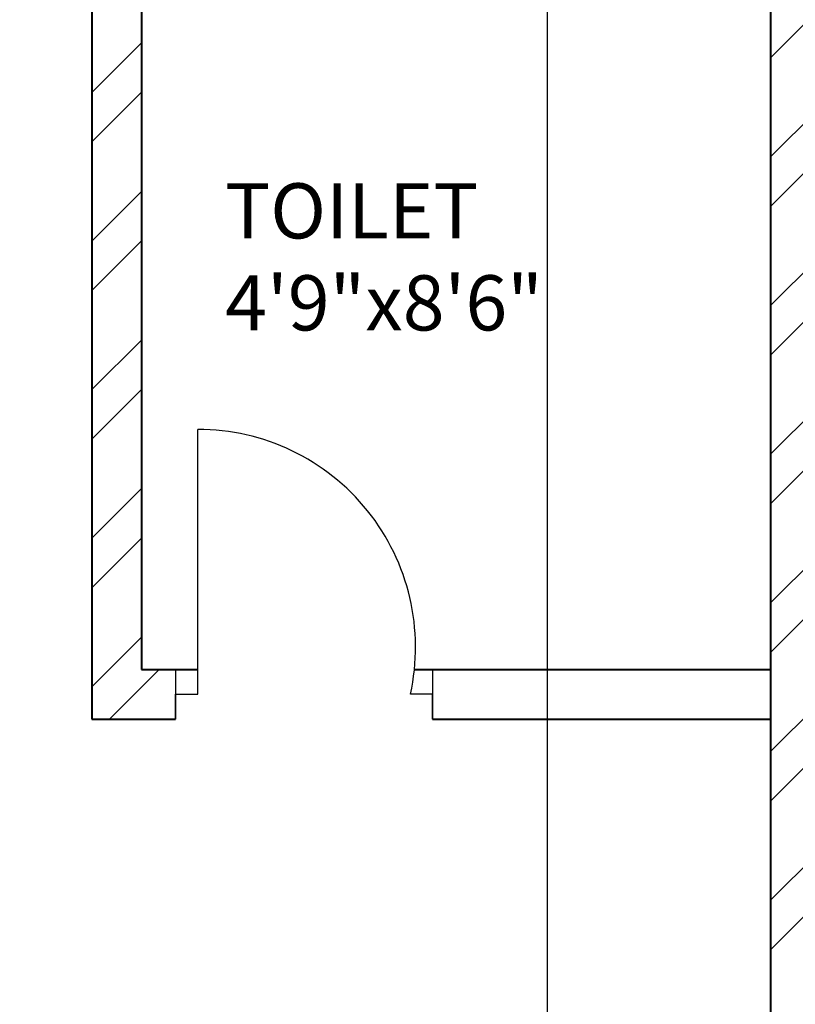
# Model space of a CAD drawing. Units: inches. Extents: x 1601 to 2297, y 1496 to 2631.
# Tile 43 of 57: x 1820 to 1891, y 2391 to 2480. Entities that reach past the tile are written whole.
import ezdxf

# ---------------------------------------------------------------- set-up
doc = ezdxf.new("R2010")
doc.units = ezdxf.units.IN
for name, color, linetype, lineweight in [('A-ANNO-DIMS', 2, 'Continuous', 18), ('A-AREA-IDEN', 7, 'Continuous', 18), ('A-DOOR', 21, 'Continuous', 25), ('A-WALL', 7, 'Continuous', 40), ('A-WALL-PATT', 215, 'Continuous', 13)]:
    doc.layers.add(name, color=color, linetype=linetype, lineweight=lineweight)
doc.styles.get("Standard").update_dxf_attribs({"font": 'arial.ttf'})
doc.dimstyles.get("Standard").update_dxf_attribs({"dimtxt": 0.18, "dimasz": 0.18, "dimexe": 0.18, "dimexo": 0.0625, "dimgap": 0.09, "dimtad": 0, "dimtih": 1, "dimtoh": 1, "dimdec": 4, "dimzin": 0, "dimdsep": 46, "dimtxsty": 'Standard', "dimcen": 0.09, "dimadec": 0, "dimazin": 0, "dimtfac": 1, "dimtdec": 4, "dimtofl": 0, "dimtmove": 0, "dimatfit": 3, "dimfxl": 1, "dimtolj": 1, "dimtzin": 0, "dimarcsym": 0})

# ---------------------------------------------------------------- blocks, each defined once
blk = doc.blocks.new('*D33')
at = {"layer": 'A-ANNO-DIMS', "color": 0, "lineweight": -2, "transparency": 16777216}
for p, q in [((1764.337, 2136.388), (1764.337, 2581.055)), ((1764.517, 2580.875), (1816.057, 2580.875)), ((1868.157, 2580.875), (1816.617, 2580.875)), ((1868.337, 2136.388), (1868.337, 2581.055))]:
    blk.add_line(p, q, dxfattribs=at)
at = {"layer": 'A-ANNO-DIMS', "color": 0, "transparency": 16777216}
for points in [[(1764.517, 2580.905), (1764.517, 2580.845), (1764.337, 2580.875)], [(1868.157, 2580.905), (1868.157, 2580.845), (1868.337, 2580.875)]]:
    blk.add_solid(points, dxfattribs=at)
at = {"layer": 'Defpoints', "color": 0, "transparency": 16777216}
for p in [(1868.337, 2580.875), (1764.337, 2136.325), (1868.337, 2136.325)]:
    blk.add_point(p, dxfattribs=at)
at = {"layer": 'A-ANNO-DIMS', "color": 0, "transparency": 16777216, "insert": (1816.337, 2580.875), "char_height": 0.18, "attachment_point": 5}
blk.add_mtext('\\A1;104', dxfattribs=at)

msp = doc.modelspace()

# ---------------------------------------------------------------- hatches: boundary and pattern name
at = {"layer": 'A-WALL-PATT'}
h = msp.add_hatch(dxfattribs=at)
h.set_pattern_fill('ANSI32', color=256)
h.paths.add_polyline_path([(1842.0336, 2528.0767), (1842.0336, 2532.3254), (1686.0373, 2532.3254), (1686.0373, 2492.9493), (1695.0373, 2492.9493), (1695.0373, 2523.3254), (1827.0373, 2523.3254), (1827.0373, 2416.8254), (1834.6225, 2416.8254), (1834.6225, 2419.0754), (1834.6225, 2421.3254), (1831.5373, 2421.3254), (1831.5373, 2523.3254), (1842.0336, 2523.3254)])
h.paths.add_polyline_path([(1695.0373, 2432.9493), (1686.0373, 2432.9493), (1686.0373, 2325.989), (1695.0373, 2325.989), (1695.0373, 2347.8254), (1827.0373, 2347.8254), (1827.0373, 2287.8254), (1823.2991, 2287.8254), (1823.2991, 2283.3254), (1847.9422, 2283.3254), (1847.9422, 2285.5754), (1847.9422, 2287.8254), (1831.5373, 2287.8254), (1831.5373, 2347.8254), (1846.9946, 2347.8254), (1846.9946, 2350.0754), (1846.9946, 2352.3254), (1695.0373, 2352.3254)])
h.paths.add_polyline_path([(1807.1169, 1573.5395), (2055.0405, 1573.5395), (2055.0405, 1610.6322), (1807.1169, 1610.6322)], flags=9)
h.paths.add_polyline_path([(1841.1631, 1712.7967), (1870.3957, 1712.7967), (1870.3957, 1731.454), (1841.1631, 1731.454)], flags=9)
h.paths.add_polyline_path([(2144.3862, 1772.185), (2191.0233, 1772.185), (2191.0233, 1790.8423), (2144.3862, 1790.8423)], flags=9)
h.paths.add_polyline_path([(2143.0128, 1827.3312), (2177.9958, 1827.3312), (2177.9958, 1845.9886), (2143.0128, 1845.9886)], flags=9)
h.paths.add_polyline_path([(2041.2439, 1833.5691), (2070.8516, 1833.5691), (2070.8516, 1852.2264), (2041.2439, 1852.2264)], flags=9)
h.paths.add_polyline_path([(2097.2791, 1947.0598), (2134.2061, 1947.0598), (2134.2061, 1965.7171), (2097.2791, 1965.7171)], flags=9)
h.paths.add_polyline_path([(2214.995, 1904.3124), (2214.995, 1942.2899), (2196.3376, 1942.2899), (2196.3376, 1904.3124)], flags=9)
h.paths.add_polyline_path([(2186.6284, 2043.8031), (2219.7935, 2043.8031), (2219.7935, 2062.4605), (2186.6284, 2062.4605)], flags=9)
h.paths.add_polyline_path([(2064.0877, 2031.616), (2097.4949, 2031.616), (2097.4949, 2050.2734), (2064.0877, 2050.2734)], flags=9)
h.paths.add_polyline_path([(1973.1349, 1986.0688), (2008.4009, 1986.0688), (2008.4009, 2004.7261), (1973.1349, 2004.7261)], flags=9)
h.paths.add_polyline_path([(1976.3676, 2106.9635), (2005.7469, 2106.9635), (2005.7469, 2125.6209), (1976.3676, 2125.6209)], flags=9)
h.paths.add_polyline_path([(1991.7852, 2180.4863), (2027.0513, 2180.4863), (2027.0513, 2199.1437), (1991.7852, 2199.1437)], flags=9)
h.paths.add_polyline_path([(2106.1801, 2187.9359), (2152.2101, 2187.9359), (2152.2101, 2206.5932), (2106.1801, 2206.5932)], flags=9)
h.paths.add_polyline_path([(2148.6686, 2262.2542), (2182.318, 2262.2542), (2182.318, 2280.9115), (2148.6686, 2280.9115)], flags=9)
h.paths.add_polyline_path([(2041.6327, 2252.8147), (2071.2405, 2252.8147), (2071.2405, 2271.4721), (2041.6327, 2271.4721)], flags=9)
h.paths.add_polyline_path([(2063.9734, 2375.4265), (2100.9004, 2375.4265), (2100.9004, 2394.0839), (2063.9734, 2394.0839)], flags=9)
h.paths.add_polyline_path([(2216.4955, 2330.9748), (2216.4955, 2370.2654), (2197.8381, 2370.2654), (2197.8381, 2330.9748)], flags=9)
h.paths.add_polyline_path([(2179.1416, 2485.8687), (2212.3067, 2485.8687), (2212.3067, 2504.5261), (2179.1416, 2504.5261)], flags=9)
h.paths.add_polyline_path([(2078.7442, 2471.1516), (2112.1514, 2471.1516), (2112.1514, 2489.809), (2078.7442, 2489.809)], flags=9)
h.paths.add_polyline_path([(1915.9631, 2329.4668), (1952.8902, 2329.4668), (1952.8902, 2348.1241), (1915.9631, 2348.1241)], flags=9)
h.paths.add_polyline_path([(1904.3189, 2499.6709), (1940.4512, 2499.6709), (1940.4512, 2518.3282), (1904.3189, 2518.3282)], flags=9)
h.paths.add_polyline_path([(1892.3665, 2100.4595), (1925.6374, 2100.4595), (1925.6374, 2119.1169), (1892.3665, 2119.1169)], flags=9)
h.paths.add_polyline_path([(1909.2984, 1805.9631), (1946.2254, 1805.9631), (1946.2254, 1824.6205), (1909.2984, 1824.6205)], flags=9)
h.paths.add_polyline_path([(1934.6056, 1658.616), (1970.738, 1658.616), (1970.738, 1677.2733), (1934.6056, 1677.2733)], flags=9)
h.paths.add_polyline_path([(1711.2052, 1789.8902), (1750.0456, 1789.8902), (1750.0456, 1808.5476), (1711.2052, 1808.5476)], flags=9)
h.paths.add_polyline_path([(1742.7874, 1854.6743), (1771.9449, 1854.6743), (1771.9449, 1873.3317), (1742.7874, 1873.3317)], flags=9)
h.paths.add_polyline_path([(1807.3592, 1997.7912), (1850.1116, 1997.7912), (1850.1116, 2016.4486), (1807.3592, 2016.4486)], flags=9)
h.paths.add_polyline_path([(1717.4579, 2237.7844), (1760.2103, 2237.7844), (1760.2103, 2256.4417), (1717.4579, 2256.4417)], flags=9)
h.paths.add_polyline_path([(1780.9285, 2324.0623), (1810.086, 2324.0623), (1810.086, 2342.7197), (1780.9285, 2342.7197)], flags=25)
h.paths.add_polyline_path([(1837.696, 2449.2024), (1866.9286, 2449.2024), (1866.9286, 2467.8598), (1837.696, 2467.8598)], flags=9)
h.paths.add_polyline_path([(1712.7752, 2484.9404), (1751.6156, 2484.9404), (1751.6156, 2503.5977), (1712.7752, 2503.5977)], flags=25)
h = msp.add_hatch(dxfattribs=at)
h.set_pattern_fill('ANSI32', color=256)
h.paths.add_polyline_path([(2230.5373, 2532.3254), (2106.0595, 2532.3254), (2106.0595, 2523.3254), (2169.0373, 2523.3254), (2169.0373, 2424.3254), (2091.3989, 2424.3254), (2091.3989, 2419.8254), (2169.0373, 2419.8254), (2169.0373, 2408.1385), (2178.0373, 2408.1385), (2178.0373, 2419.8254), (2181.0581, 2419.8254), (2181.0581, 2422.0754), (2181.0581, 2424.3254), (2178.0373, 2424.3254), (2178.0373, 2523.3254), (2226.0373, 2523.3254), (2226.0373, 2424.3254), (2206.6251, 2424.3254), (2206.6251, 2419.8254), (2226.0373, 2419.8254), (2226.0373, 2299.8254), (2226.0373, 2295.3254), (2178.0373, 2295.3254), (2178.0373, 2312.1385), (2169.0373, 2312.1385), (2169.0373, 2295.3254), (2130.0373, 2295.3254), (2130.0373, 2279.1364), (2128.0593, 2279.1364), (2128.0593, 2274.6364), (2130.0373, 2274.6364), (2130.0373, 2260.7505), (2134.5373, 2260.7505), (2134.5373, 2290.8254), (2226.0373, 2290.8254), (2226.0373, 2279.2475), (2230.5373, 2279.2475), (2230.5373, 2347.8254)])
h.paths.add_polyline_path([(2070.0595, 2532.3254), (2031.0373, 2532.3254), (2031.0373, 2466.3254), (2003.9878, 2466.3254), (2003.9878, 2457.3254), (2031.0373, 2457.3254), (2031.0373, 2419.8254), (2031.0373, 2373.1914), (2035.5373, 2373.1914), (2035.5373, 2419.8254), (2047.3393, 2419.8254), (2047.3393, 2424.3254), (2035.5373, 2424.3254), (2035.5373, 2523.3254), (2070.0595, 2523.3254), (2070.0595, 2527.8254)])
h.paths.add_polyline_path([(1893.0373, 2532.3254), (1866.0336, 2532.3254), (1866.0336, 2523.3254), (1888.5373, 2523.3254), (1888.5373, 2347.8254), (1893.0373, 2347.8254), (1893.0373, 2457.3254), (1907.9878, 2457.3254), (1907.9878, 2466.3254), (1893.0373, 2466.3254)])
h = msp.add_hatch(dxfattribs=at)
h.set_pattern_fill('ANSI32', color=256)
h.paths.add_polyline_path([(1973.9371, 2211.3254), (1893.0373, 2211.3254), (1893.0373, 2287.8254), (1884.6167, 2287.8254), (1884.6167, 2285.5754), (1884.6167, 2283.3254), (1888.5373, 2283.3254), (1888.5373, 2145.3254), (1695.0373, 2145.3254), (1695.0373, 2173.8724), (1690.5373, 2173.8724), (1686.0373, 2173.8724), (1686.0373, 2136.3254), (1722.5687, 2136.3254), (1722.5687, 2117.4352), (1731.5687, 2117.4352), (1731.5687, 2136.3254), (1893.0373, 2136.3254), (1893.0373, 2202.3254), (1959.0373, 2202.3254), (1959.0373, 2182.1303), (1968.0373, 2182.1303), (1968.0373, 2202.3254), (1973.9371, 2202.3254)])
h.paths.add_polyline_path([(2094.0373, 2274.6364), (2096.4294, 2274.6364), (2096.4294, 2276.8864), (2096.4294, 2279.1364), (2094.0373, 2279.1364), (2094.0373, 2290.8254), (2094.0373, 2295.3254), (2089.5373, 2295.3254), (2089.5373, 2230.8254), (2035.5373, 2230.8254), (2035.5373, 2299.8254), (2031.0373, 2299.8254), (2031.0373, 2211.3254), (2023.0065, 2211.3254), (2023.0065, 2202.3254), (2031.0373, 2202.3254), (2031.0373, 2140.8254), (1968.0373, 2140.8254), (1968.0373, 2145.9106), (1963.5373, 2145.9106), (1959.0373, 2145.9106), (1959.0373, 2116.839), (1963.5373, 2116.839), (1968.0373, 2116.839), (1968.0373, 2131.8254), (2031.0373, 2131.8254), (2031.0373, 2094.3254), (2031.0373, 2085.3254), (2031.0373, 2056.8254), (1968.0373, 2056.8254), (1968.0373, 2070.4947), (1963.5373, 2070.4947), (1959.0373, 2070.4947), (1959.0373, 2040.3029), (1968.0373, 2040.3029), (1968.0373, 2047.8254), (2031.0373, 2047.8254), (2031.0373, 1983.3254), (2031.0373, 1978.8254), (2021.1979, 1978.8254), (2021.1979, 1974.3254), (2031.0373, 1974.3254), (2031.0373, 1954.3528), (2035.5373, 1954.3528), (2035.5373, 1974.3254), (2035.5373, 1981.8254), (2055.5513, 1981.8254), (2055.5513, 1986.3254), (2035.5373, 1986.3254), (2035.5373, 2047.8254), (2040.0373, 2047.8254), (2040.0373, 2085.3254), (2040.0373, 2094.3254), (2040.0373, 2140.8254), (2035.5373, 2140.8254), (2035.5373, 2226.3254), (2089.5373, 2226.3254), (2094.0373, 2226.3254)])
h.paths.add_polyline_path([(2226.0373, 2230.8254), (2134.5373, 2230.8254), (2134.5373, 2233.5437), (2130.0373, 2233.5437), (2130.0373, 2226.3254), (2134.5373, 2226.3254), (2226.0373, 2226.3254)])
h.paths.add_polyline_path([(1807.1169, 1573.5395), (2055.0405, 1573.5395), (2055.0405, 1610.6322), (1807.1169, 1610.6322)], flags=9)
h.paths.add_polyline_path([(1841.1631, 1712.7967), (1870.3957, 1712.7967), (1870.3957, 1731.454), (1841.1631, 1731.454)], flags=9)
h.paths.add_polyline_path([(2144.3862, 1772.185), (2191.0233, 1772.185), (2191.0233, 1790.8423), (2144.3862, 1790.8423)], flags=9)
h.paths.add_polyline_path([(2143.0128, 1827.3312), (2177.9958, 1827.3312), (2177.9958, 1845.9886), (2143.0128, 1845.9886)], flags=9)
h.paths.add_polyline_path([(2041.2439, 1833.5691), (2070.8516, 1833.5691), (2070.8516, 1852.2264), (2041.2439, 1852.2264)], flags=9)
h.paths.add_polyline_path([(2097.2791, 1947.0598), (2134.2061, 1947.0598), (2134.2061, 1965.7171), (2097.2791, 1965.7171)], flags=9)
h.paths.add_polyline_path([(2214.995, 1904.3124), (2214.995, 1942.2899), (2196.3376, 1942.2899), (2196.3376, 1904.3124)], flags=9)
h.paths.add_polyline_path([(2186.6284, 2043.8031), (2219.7935, 2043.8031), (2219.7935, 2062.4605), (2186.6284, 2062.4605)], flags=9)
h.paths.add_polyline_path([(2064.0877, 2031.616), (2097.4949, 2031.616), (2097.4949, 2050.2734), (2064.0877, 2050.2734)], flags=9)
h.paths.add_polyline_path([(1973.1349, 1986.0688), (2008.4009, 1986.0688), (2008.4009, 2004.7261), (1973.1349, 2004.7261)], flags=25)
h.paths.add_polyline_path([(1976.3676, 2106.9635), (2005.7469, 2106.9635), (2005.7469, 2125.6209), (1976.3676, 2125.6209)], flags=25)
h.paths.add_polyline_path([(1991.7852, 2180.4863), (2027.0513, 2180.4863), (2027.0513, 2199.1437), (1991.7852, 2199.1437)], flags=25)
h.paths.add_polyline_path([(2106.1801, 2187.9359), (2152.2101, 2187.9359), (2152.2101, 2206.5932), (2106.1801, 2206.5932)], flags=9)
h.paths.add_polyline_path([(2148.6686, 2262.2542), (2182.318, 2262.2542), (2182.318, 2280.9115), (2148.6686, 2280.9115)], flags=9)
h.paths.add_polyline_path([(2041.6327, 2252.8147), (2071.2405, 2252.8147), (2071.2405, 2271.4721), (2041.6327, 2271.4721)], flags=25)
h.paths.add_polyline_path([(2063.9734, 2375.4265), (2100.9004, 2375.4265), (2100.9004, 2394.0839), (2063.9734, 2394.0839)], flags=9)
h.paths.add_polyline_path([(2216.4955, 2330.9748), (2216.4955, 2370.2654), (2197.8381, 2370.2654), (2197.8381, 2330.9748)], flags=9)
h.paths.add_polyline_path([(2179.1416, 2485.8687), (2212.3067, 2485.8687), (2212.3067, 2504.5261), (2179.1416, 2504.5261)], flags=9)
h.paths.add_polyline_path([(2078.7442, 2471.1516), (2112.1514, 2471.1516), (2112.1514, 2489.809), (2078.7442, 2489.809)], flags=9)
h.paths.add_polyline_path([(1915.9631, 2329.4668), (1952.8902, 2329.4668), (1952.8902, 2348.1241), (1915.9631, 2348.1241)], flags=9)
h.paths.add_polyline_path([(1904.3189, 2499.6709), (1940.4512, 2499.6709), (1940.4512, 2518.3282), (1904.3189, 2518.3282)], flags=9)
h.paths.add_polyline_path([(1892.3665, 2100.4595), (1925.6374, 2100.4595), (1925.6374, 2119.1169), (1892.3665, 2119.1169)], flags=9)
h.paths.add_polyline_path([(1909.2984, 1805.9631), (1946.2254, 1805.9631), (1946.2254, 1824.6205), (1909.2984, 1824.6205)], flags=9)
h.paths.add_polyline_path([(1934.6056, 1658.616), (1970.738, 1658.616), (1970.738, 1677.2733), (1934.6056, 1677.2733)], flags=9)
h.paths.add_polyline_path([(1711.2052, 1789.8902), (1750.0456, 1789.8902), (1750.0456, 1808.5476), (1711.2052, 1808.5476)], flags=9)
h.paths.add_polyline_path([(1742.7874, 1854.6743), (1771.9449, 1854.6743), (1771.9449, 1873.3317), (1742.7874, 1873.3317)], flags=9)
h.paths.add_polyline_path([(1807.3592, 1997.7912), (1850.1116, 1997.7912), (1850.1116, 2016.4486), (1807.3592, 2016.4486)], flags=9)
h.paths.add_polyline_path([(1717.4579, 2237.7844), (1760.2103, 2237.7844), (1760.2103, 2256.4417), (1717.4579, 2256.4417)], flags=25)
h.paths.add_polyline_path([(1780.9285, 2324.0623), (1810.086, 2324.0623), (1810.086, 2342.7197), (1780.9285, 2342.7197)], flags=9)
h.paths.add_polyline_path([(1837.696, 2449.2024), (1866.9286, 2449.2024), (1866.9286, 2467.8598), (1837.696, 2467.8598)], flags=9)
h.paths.add_polyline_path([(1712.7752, 2484.9404), (1751.6156, 2484.9404), (1751.6156, 2503.5977), (1712.7752, 2503.5977)], flags=9)
h = msp.add_hatch(dxfattribs=at)
h.set_pattern_fill('ANSI32', color=256)
h.paths.add_polyline_path([(2230.5373, 1861.8254), (2182.5373, 1861.8254), (2182.5373, 1885.3637), (2178.0373, 1885.3637), (2178.0373, 1861.8254), (2166.0373, 1861.8254), (2134.5373, 1861.8254), (2130.0373, 1861.8254), (2130.0373, 1841.4682), (2126.8833, 1841.4682), (2126.8833, 1836.9682), (2130.0373, 1836.9682), (2130.0373, 1822.7302), (2134.5373, 1822.7302), (2134.5373, 1857.3254), (2166.0373, 1857.3254), (2226.0373, 1857.3254), (2226.0373, 1846.1155), (2230.5373, 1846.1155)])
h.paths.add_polyline_path([(2226.0373, 1797.3254), (2134.5373, 1797.3254), (2134.5373, 1800.6636), (2132.2873, 1800.6636), (2130.0373, 1800.6636), (2130.0373, 1797.3254), (2130.0373, 1792.8254), (2167.7264, 1792.8254), (2226.0373, 1792.8254)])
h.paths.add_polyline_path([(2230.5373, 1822.1155), (2226.0373, 1822.1155), (2226.0373, 1760.8563), (2230.5373, 1760.8563)])
h.paths.add_polyline_path([(2230.5373, 1700.8563), (2226.0373, 1700.8563), (2226.0373, 1644.3254), (2140.2517, 1644.3254), (2140.2517, 1635.3254), (2230.5373, 1635.3254)])
h.paths.add_polyline_path([(2080.2517, 1639.8254), (2080.2517, 1644.3254), (2035.5373, 1644.3254), (2035.5373, 1792.8254), (2094.0373, 1792.8254), (2094.0373, 1797.3254), (2094.0373, 1836.9682), (2097.1057, 1836.9682), (2097.1057, 1839.2182), (2097.1057, 1841.4682), (2094.0373, 1841.4682), (2094.0373, 1862.2276), (2089.5373, 1862.2276), (2089.5373, 1797.3254), (2035.5373, 1797.3254), (2035.5373, 1857.3254), (2035.5373, 1885.0916), (2031.0373, 1885.0916), (2031.0373, 1710.3254), (2012.329, 1710.3254), (2012.329, 1701.3254), (2031.0373, 1701.3254), (2031.0373, 1644.3254), (2031.0373, 1635.3254), (2080.2517, 1635.3254)])
h.paths.add_polyline_path([(1836.0373, 1653.2033), (1842.6171, 1653.2033), (1842.6171, 1657.7033), (1842.6171, 1662.2033), (1831.5373, 1662.2033), (1831.5373, 1764.2033), (1835.3881, 1764.2033), (1835.3881, 1766.4533), (1835.3881, 1768.7033), (1831.5373, 1768.7033), (1827.0373, 1768.7033), (1827.0373, 1662.2033), (1827.0373, 1635.3254), (1836.0373, 1635.3254)])
h.paths.add_polyline_path([(1893.0373, 1701.3254), (1907.193, 1701.3254), (1907.193, 1705.8254), (1907.193, 1710.3254), (1893.0373, 1710.3254), (1893.0373, 1819.8254), (1882.6444, 1819.8254), (1882.6444, 1817.5754), (1882.6444, 1815.3254), (1888.5373, 1815.3254), (1888.5373, 1662.2033), (1884.0373, 1662.2033), (1866.6171, 1662.2033), (1866.6171, 1653.2033), (1882.391, 1653.2033), (1884.0373, 1653.2033), (1884.0373, 1635.3254), (1893.0373, 1635.3254)])
h.paths.add_polyline_path([(1739.3335, 1639.8254), (1739.3335, 1644.3254), (1695.0373, 1644.3254), (1695.0373, 1702.0135), (1690.5373, 1702.0135), (1686.0373, 1702.0135), (1686.0373, 1635.3254), (1739.3335, 1635.3254)])
h.paths.add_polyline_path([(1827.0373, 1644.3254), (1799.3335, 1644.3254), (1799.3335, 1635.3254), (1827.0373, 1635.3254)])
h.paths.add_polyline_path([(1695.0373, 1815.3254), (1849.2759, 1815.3254), (1849.2759, 1819.8254), (1807.5373, 1819.8254), (1807.5373, 1879.8254), (1851.1533, 1879.8254), (1851.1533, 1882.0754), (1851.1533, 1884.3254), (1799.3405, 1884.3254), (1799.3405, 1882.0754), (1799.3405, 1879.8254), (1803.0373, 1879.8254), (1803.0373, 1819.8254), (1695.0373, 1819.8254), (1695.0373, 1835.0458), (1690.5373, 1835.0458), (1686.0373, 1835.0458), (1686.0373, 1766.1753), (1695.0373, 1766.1753)])
h.paths.add_polyline_path([(1775.8157, 1884.3254), (1695.0373, 1884.3254), (1695.0373, 1912.9526), (1690.5373, 1912.9526), (1686.0373, 1912.9526), (1686.0373, 1859.0458), (1695.0373, 1859.0458), (1695.0373, 1879.8254), (1775.8157, 1879.8254)])
h.paths.add_polyline_path([(1893.0373, 2031.3254), (1731.5687, 2031.3254), (1731.5687, 2057.4352), (1722.5687, 2057.4352), (1722.5687, 2031.3254), (1686.0373, 2031.3254), (1686.0373, 1972.9526), (1695.0373, 1972.9526), (1695.0373, 2022.3254), (1888.5373, 2022.3254), (1888.5373, 1884.3254), (1883.4996, 1884.3254), (1883.4996, 1879.8254), (1893.0373, 1879.8254), (1893.0373, 1974.3254), (1976.6199, 1974.3254), (1976.6199, 1978.8254), (1968.0373, 1978.8254), (1968.0373, 1983.3254), (1968.0373, 2008.4756), (1963.5373, 2008.4756), (1959.0373, 2008.4756), (1959.0373, 1983.3254), (1893.0373, 1983.3254)])
h.paths.add_polyline_path([(2230.5373, 2140.4745), (2226.0373, 2140.4745), (2226.0373, 2094.3254), (2040.0373, 2094.3254), (2040.0373, 2085.3254), (2178.0373, 2085.3254), (2178.0373, 2065.6965), (2182.5373, 2065.6965), (2182.5373, 2085.3254), (2226.0373, 2085.3254), (2226.0373, 1986.3254), (2211.2679, 1986.3254), (2211.2679, 1981.8254), (2230.5373, 1981.8254)])
h.paths.add_polyline_path([(2187.6292, 1986.3254), (2182.5373, 1986.3254), (2182.5373, 2029.6965), (2178.0373, 2029.6965), (2178.0373, 1986.3254), (2099.05, 1986.3254), (2099.05, 1981.8254), (2178.0373, 1981.8254), (2178.0373, 1969.3637), (2182.5373, 1969.3637), (2182.5373, 1981.8254), (2187.6292, 1981.8254), (2187.6292, 1984.0754)])
h.paths.add_polyline_path([(1807.1169, 1573.5395), (2055.0405, 1573.5395), (2055.0405, 1610.6322), (1807.1169, 1610.6322)], flags=9)
h.paths.add_polyline_path([(1841.1631, 1712.7967), (1870.3957, 1712.7967), (1870.3957, 1731.454), (1841.1631, 1731.454)], flags=9)
h.paths.add_polyline_path([(2144.3862, 1772.185), (2191.0233, 1772.185), (2191.0233, 1790.8423), (2144.3862, 1790.8423)], flags=9)
h.paths.add_polyline_path([(2143.0128, 1827.3312), (2177.9958, 1827.3312), (2177.9958, 1845.9886), (2143.0128, 1845.9886)], flags=25)
h.paths.add_polyline_path([(2041.2439, 1833.5691), (2070.8516, 1833.5691), (2070.8516, 1852.2264), (2041.2439, 1852.2264)], flags=25)
h.paths.add_polyline_path([(2097.2791, 1947.0598), (2134.2061, 1947.0598), (2134.2061, 1965.7171), (2097.2791, 1965.7171)], flags=9)
h.paths.add_polyline_path([(2214.995, 1904.3124), (2214.995, 1942.2899), (2196.3376, 1942.2899), (2196.3376, 1904.3124)], flags=9)
h.paths.add_polyline_path([(2186.6284, 2043.8031), (2219.7935, 2043.8031), (2219.7935, 2062.4605), (2186.6284, 2062.4605)], flags=25)
h.paths.add_polyline_path([(2064.0877, 2031.616), (2097.4949, 2031.616), (2097.4949, 2050.2734), (2064.0877, 2050.2734)], flags=25)
h.paths.add_polyline_path([(1973.1349, 1986.0688), (2008.4009, 1986.0688), (2008.4009, 2004.7261), (1973.1349, 2004.7261)], flags=9)
h.paths.add_polyline_path([(1976.3676, 2106.9635), (2005.7469, 2106.9635), (2005.7469, 2125.6209), (1976.3676, 2125.6209)], flags=9)
h.paths.add_polyline_path([(1991.7852, 2180.4863), (2027.0513, 2180.4863), (2027.0513, 2199.1437), (1991.7852, 2199.1437)], flags=9)
h.paths.add_polyline_path([(2106.1801, 2187.9359), (2152.2101, 2187.9359), (2152.2101, 2206.5932), (2106.1801, 2206.5932)], flags=9)
h.paths.add_polyline_path([(2148.6686, 2262.2542), (2182.318, 2262.2542), (2182.318, 2280.9115), (2148.6686, 2280.9115)], flags=9)
h.paths.add_polyline_path([(2041.6327, 2252.8147), (2071.2405, 2252.8147), (2071.2405, 2271.4721), (2041.6327, 2271.4721)], flags=9)
h.paths.add_polyline_path([(2063.9734, 2375.4265), (2100.9004, 2375.4265), (2100.9004, 2394.0839), (2063.9734, 2394.0839)], flags=9)
h.paths.add_polyline_path([(2216.4955, 2330.9748), (2216.4955, 2370.2654), (2197.8381, 2370.2654), (2197.8381, 2330.9748)], flags=9)
h.paths.add_polyline_path([(2179.1416, 2485.8687), (2212.3067, 2485.8687), (2212.3067, 2504.5261), (2179.1416, 2504.5261)], flags=9)
h.paths.add_polyline_path([(2078.7442, 2471.1516), (2112.1514, 2471.1516), (2112.1514, 2489.809), (2078.7442, 2489.809)], flags=9)
h.paths.add_polyline_path([(1915.9631, 2329.4668), (1952.8902, 2329.4668), (1952.8902, 2348.1241), (1915.9631, 2348.1241)], flags=9)
h.paths.add_polyline_path([(1904.3189, 2499.6709), (1940.4512, 2499.6709), (1940.4512, 2518.3282), (1904.3189, 2518.3282)], flags=9)
h.paths.add_polyline_path([(1892.3665, 2100.4595), (1925.6374, 2100.4595), (1925.6374, 2119.1169), (1892.3665, 2119.1169)], flags=9)
h.paths.add_polyline_path([(1909.2984, 1805.9631), (1946.2254, 1805.9631), (1946.2254, 1824.6205), (1909.2984, 1824.6205)], flags=9)
h.paths.add_polyline_path([(1934.6056, 1658.616), (1970.738, 1658.616), (1970.738, 1677.2733), (1934.6056, 1677.2733)], flags=9)
h.paths.add_polyline_path([(1711.2052, 1789.8902), (1750.0456, 1789.8902), (1750.0456, 1808.5476), (1711.2052, 1808.5476)], flags=25)
h.paths.add_polyline_path([(1742.7874, 1854.6743), (1771.9449, 1854.6743), (1771.9449, 1873.3317), (1742.7874, 1873.3317)], flags=25)
h.paths.add_polyline_path([(1807.3592, 1997.7912), (1850.1116, 1997.7912), (1850.1116, 2016.4486), (1807.3592, 2016.4486)], flags=25)
h.paths.add_polyline_path([(1717.4579, 2237.7844), (1760.2103, 2237.7844), (1760.2103, 2256.4417), (1717.4579, 2256.4417)], flags=9)
h.paths.add_polyline_path([(1780.9285, 2324.0623), (1810.086, 2324.0623), (1810.086, 2342.7197), (1780.9285, 2342.7197)], flags=9)
h.paths.add_polyline_path([(1837.696, 2449.2024), (1866.9286, 2449.2024), (1866.9286, 2467.8598), (1837.696, 2467.8598)], flags=9)
h.paths.add_polyline_path([(1712.7752, 2484.9404), (1751.6156, 2484.9404), (1751.6156, 2503.5977), (1712.7752, 2503.5977)], flags=9)

# ---------------------------------------------------------------- linework, layer by layer
at = {"layer": 'A-DOOR'}
for p, q in [((1836.6225, 2419.0754), (1836.6225, 2443.0754)), ((1834.6225, 2421.3254), (1834.6225, 2416.8254)), ((1857.9041, 2421.3254), (1857.9041, 2416.8254)), ((1834.6225, 2416.8254), (1834.6225, 2419.0754)), ((1834.6225, 2419.0754), (1836.6225, 2419.0754)), ((1857.9041, 2419.0754), (1855.9041, 2419.0754)), ((1857.9041, 2416.8254), (1857.9041, 2419.0754))]:
    msp.add_line(p, q, dxfattribs=at)
msp.add_arc((1836.6225, 2423.3299), 19.7454, 347.556809, 90, dxfattribs=at)
at = {"layer": 'A-WALL'}
for p, q in [((1827.0373, 2523.3254), (1827.0373, 2416.8254)), ((1831.5373, 2523.3254), (1831.5373, 2421.3254)), ((1888.5373, 2523.3254), (1888.5373, 2347.8254)), ((1831.5373, 2421.3254), (1836.6225, 2421.3254)), ((1856.2659, 2421.3254), (1888.5373, 2421.3254)), ((1827.0373, 2416.8254), (1834.6225, 2416.8254)), ((1857.9041, 2416.8254), (1888.5373, 2416.8254))]:
    msp.add_line(p, q, dxfattribs=at)

# ---------------------------------------------------------------- texts
at = {"layer": 'A-AREA-IDEN', "insert": (1839.1097, 2465.3751), "char_height": 5, "attachment_point": 1}
msp.add_mtext_dynamic_manual_height_columns('TOILET\\P4\'9"x8\'6"', width=44.81079, gutter_width=12.5, heights=[0], dxfattribs=at)

# ---------------------------------------------------------------- dimensions: what is measured, and where the dimension line sits
at = {"layer": 'A-ANNO-DIMS'}
dim = msp.add_linear_dim(base=(1868.3371, 2580.8754), p1=(1764.3371, 2136.3254), p2=(1868.3371, 2136.3254), dimstyle='Standard', override={"dimdec": 0, "dimlfac": 1, "dimrnd": 0, "dimzin": 0, "dimdsep": 46, "dimlunit": 2}, dxfattribs=at)
dim.commit()
dim.dimension.update_dxf_attribs({"geometry": '*D33', "text_midpoint": (1816.3371, 2580.8754)})

doc.saveas('drawing.dxf')
